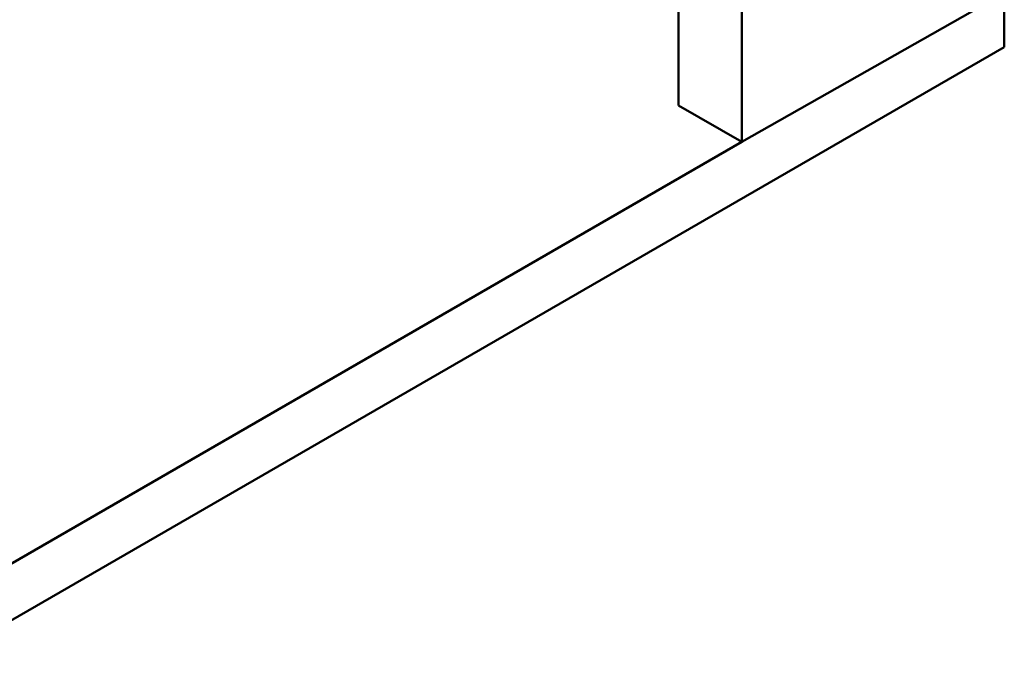
# Model space of a CAD drawing. Units: inches. Extents: x 5770 to 11891, y 3254 to 6808.
# Tile 4 of 15: x 5976 to 6133, y 3254 to 3357. Entities that reach past the tile are written whole.
import ezdxf

# ---------------------------------------------------------------- set-up
doc = ezdxf.new("R2010")
doc.units = ezdxf.units.IN
doc.layers.add('A-WALL', color=7, linetype='Continuous', lineweight=50)

msp = doc.modelspace()

# ---------------------------------------------------------------- linework, layer by layer
at = {"layer": 'A-WALL'}
for p, q in [((6132.52, 3448.83), (6132.52, 3352.22)), ((6080.71, 3430.94), (6080.71, 3342.94)), ((6090.78, 3425.13), (6090.78, 3337.13)), ((6132.52, 3360.83), (6090.78, 3337.13)), ((6132.52, 3352.22), (5962.44, 3254.03)), ((6080.71, 3342.94), (6090.78, 3337.13)), ((6090.78, 3337.13), (5962.44, 3263.03))]:
    msp.add_line(p, q, dxfattribs=at)

doc.saveas('drawing.dxf')
